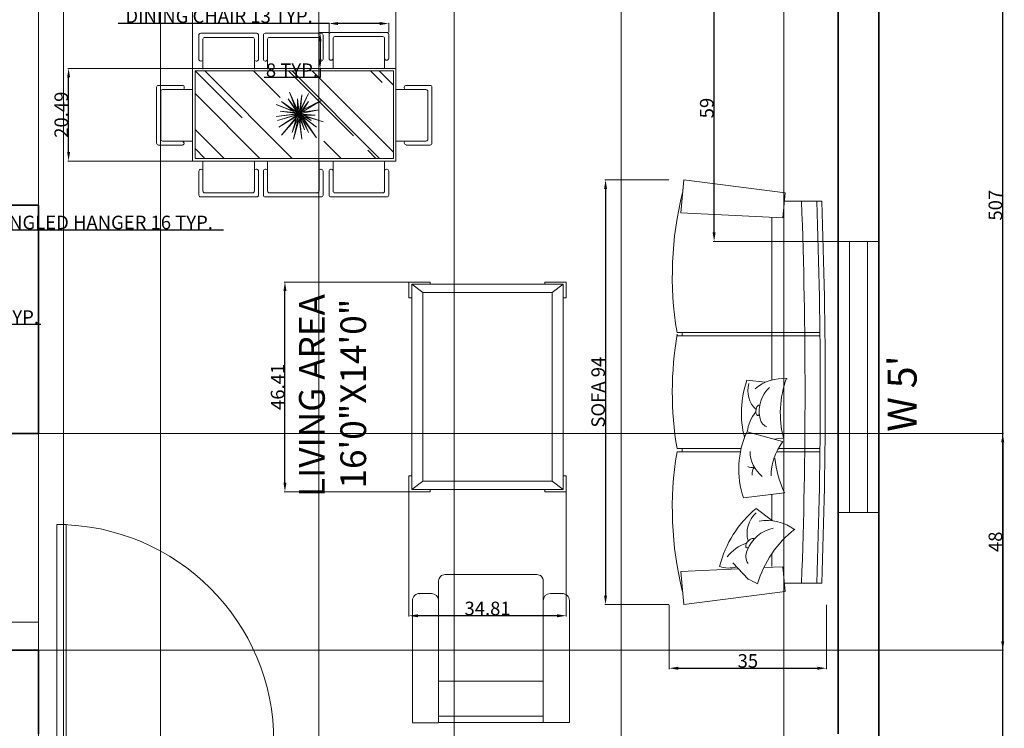
# Model space of a CAD drawing. Units: feet. Extents: x -297 to 770, y -228 to 625.
# Tile 5 of 14: x 552 to 770, y -62 to 95. Entities that reach past the tile are written whole.
import ezdxf

# ---------------------------------------------------------------- set-up
doc = ezdxf.new("R2010")
doc.units = ezdxf.units.FT
doc.header["$MEASUREMENT"] = 0
for name, color, linetype, lineweight in [('A-ANNO-DIMS', 2, 'Continuous', 18), ('A-ANNO-TEXT', 7, 'Continuous', 18), ('A-AREA-IDEN', 7, 'Continuous', 25), ('A-FURN', 8, 'Continuous', 18), ('A-WALL', 7, 'Continuous', 35), ('doors', 30, 'Continuous', 18), ('windows', 30, 'Continuous', 18)]:
    doc.layers.add(name, color=color, linetype=linetype, lineweight=lineweight)
doc.styles.add('Annotative', font='arial.ttf')
doc.styles.get("Standard").update_dxf_attribs({"font": 'arial.ttf'})
doc.dimstyles.get("Standard").update_dxf_attribs({"dimtxt": 3, "dimasz": 2, "dimexe": 0.18, "dimexo": 0.0625, "dimgap": 0.09, "dimtad": 1, "dimtoh": 1, "dimdec": 1, "dimzin": 0, "dimdsep": 46, "dimlunit": 3, "dimtxsty": 'Standard', "dimcen": 0, "dimclre": 256, "dimadec": 0, "dimazin": 0, "dimtfac": 1, "dimtdec": 1, "dimtofl": 0, "dimtmove": 0, "dimatfit": 3, "dimfxl": 1, "dimtolj": 1, "dimtzin": 0, "dimlwe": -1, "dimarcsym": 0})

# ---------------------------------------------------------------- blocks, each defined once
blk = doc.blocks.new('*U4')
for p, q in [((0, 0), (0, 6)), ((40, 0), (40, 6))]:
    blk.add_line(p, q)
blk.add_lwpolyline([(0, 0), (0, -40), (1.75, -40), (1.75, 0)], close=True)
blk.add_arc((0, 0), 40, 270, 0)
blk = doc.blocks.new('*U5')
for p, q in [((-40, 0), (-40, 6)), ((0, 0), (0, 6))]:
    blk.add_line(p, q)
blk.add_lwpolyline([(0, 0), (0, -40), (-1.75, -40), (-1.75, 0)], close=True)
blk.add_arc((0, 0), 40, 180, 270)
blk = doc.blocks.new('ММ404_2555х920')
for p, q in [((-1150, -20.9), (-1150, -245.9)), ((-360, -32.1), (-360, -892.6)), ((-340, -31.8), (-340, -892.6)), ((340, -31.8), (340, -283.8)), ((360, -32.1), (360, -293.8)), ((1150, -20.9), (1150, -245.9)), ((-1199.8, -241.6), (-1278.3, -852.1)), ((-1050.4, -254.7), (-1199.8, -241.6)), ((-1050.4, -254.7), (-1079.1, -869.5)), ((237.8, -471.1), (297.3, -256.4)), ((636.4, -491.8), (605.4, -246.1)), ((1050.4, -254.7), (1199.8, -241.6)), ((1050.4, -254.7), (1055.7, -369.5)), ((1199.8, -241.6), (1278.3, -852.1)), ((-1050, -320.9), (-73.8, -320.9)), ((614.8, -320.9), (774.2, -320.9)), ((699.6, -415.1), (774.5, -318.5)), ((971.6, -320.9), (1050, -320.9)), ((-72, -471.4), (-59.5, -361)), ((1026.9, -555.9), (1126.3, -464.2)), ((340, -506.7), (340, -892.6)), ((360, -511.1), (360, -892.6)), ((1062.9, -522.7), (1079.1, -869.5)), ((-1278.3, -852.1), (-1079.1, -869.5)), ((-360, -862.6), (-340, -862.6)), ((360, -862.6), (340, -862.6)), ((1278.3, -852.1), (1079.1, -869.5))]:
    blk.add_line(p, q)
for centre, radius, start, end in [((0, -31584.1), 31584.1, 87.91336, 92.08664), ((0, -31614.1), 31584.1, 87.91336, 92.08664), ((0, -31705.7), 31584.1, 87.91336, 92.08664), ((125.1, 326.1), 596.6, 249.48999, 284.83699), ((171.1, -255.4), 253.6, 174.21375, 221.17742), ((1051.5, -351.2), 279, 142.88134, 189.84501), ((1340.9, 221.6), 656.3, 218.15758, 253.50458), ((531.3, -258.2), 253.6, 178.2735, 191.49113), ((507.2, 23.9), 350.1, 233.17631, 269.54807), ((320.7, 386.4), 693.6, 276.31042, 294.23297), ((115.3, -200.3), 197.4, 223.39126, 280.29978), ((142.6, -321.2), 73.7, 276.25479, 334.78386), ((1030.6, -267.5), 217.1, 192.05885, 248.96737), ((85.8, -397.3), 8.22, 169.68836, 209.59655), ((85.8, -397.3), 8.22, 157.49693, 169.68836), ((98.3, -390.2), 22.6, 209.59655, 233.34145), ((108.2, -376.8), 39.2, 233.34145, 248.09558), ((117.3, -354.4), 63.4, 248.09558, 259.68836), ((122.4, -394.6), 22.6, 286.03528, 309.78017), ((119.1, -412.7), 22.6, 29.59655, 45.24399), ((131.6, -405.6), 8.22, 309.78017, 349.68836), ((131.6, -405.6), 8.22, 349.68836, 29.59655), ((353.1, -253.5), 199.6, 271.07138, 320.43697), ((1206.8, 1.3), 656.3, 219.38257, 256.10059), ((1388.4, -559.9), 279, 146.94109, 159.93675), ((125.1, 91.8), 596.6, 250.71498, 284.37724), ((-8.8, -312.1), 154, 253.94738, 317.31928), ((117.3, -354.4), 63.4, 259.68836, 271.28115), ((117.8, -378.6), 39.2, 271.28115, 286.03528), ((260.5, -254), 216.6, 229.12407, 264.09953), ((462.6, 9.9), 531, 244.94988, 289.10664), ((405.8, -444.2), 47.7, 332.00647, 20.30172), ((493.1, -362.9), 77.4, 236.70882, 274.52537), ((850, -301.6), 169.4, 222.61497, 285.98687), ((890.2, -435.7), 9.04, 138.35595, 178.26414), ((906, -436.2), 24.9, 178.26414, 202.00904), ((923, -429.3), 43.2, 202.00904, 216.76317), ((890.2, -435.7), 9.04, 126.16453, 138.35595), ((944.3, -413.4), 69.8, 216.76317, 228.35595), ((944.3, -413.4), 69.8, 228.35595, 239.94874), ((1136.3, -401), 238.2, 197.79166, 232.76712), ((931, -436.4), 43.2, 239.94874, 254.70287), ((928.5, -469.7), 9.04, 318.35595, 358.26414), ((912.6, -469.3), 24.9, 358.26414, 13.91158), ((987, -396.7), 81.1, 244.92238, 303.45145), ((926.1, -454.1), 24.9, 254.70287, 278.44776), ((928.5, -469.7), 9.04, 278.44776, 318.35595), ((896.2, -581.2), 162.4, 340.38592, 16.76075), ((-700, 1135.7), 2056.7, 255.87327, 279.51559), ((700, 1135.7), 2056.7, 260.48441, 284.12673), ((0, 1135.7), 2056.7, 260.20182, 279.51559)]:
    blk.add_arc(centre, radius, start, end)
blk = doc.blocks.new('WIN-5FT')
for p, q in [((60, 6.5), (0, 6.5)), ((60, 2.5), (0, 2.5))]:
    blk.add_line(p, q)
blk.add_lwpolyline([(60, 0), (60, 9), (0, 9), (0, 0)], close=True)
blk = doc.blocks.new('DINING-CHAIR')
for p, q in [((0.91, 1.32), (0.91, 7.97)), ((12.3, 7.97), (12.3, 1.32)), ((0, 0.41), (0, 5.72)), ((0.5, 6.13), (0.41, 6.13)), ((12.8, 6.13), (12.71, 6.13)), ((13.21, 5.72), (13.21, 0.41)), ((12.8, 0), (0.41, 0)), ((11.89, 0.91), (1.32, 0.91))]:
    blk.add_line(p, q)
for centre, start, end in [((0.41, 5.72), 90, 180), ((0.5, 5.72), 0, 90), ((12.71, 5.72), 90, 180), ((12.8, 5.72), 0, 90), ((0.41, 0.41), 180, 270), ((1.32, 1.32), 180, 270), ((11.89, 1.32), 270, 0), ((12.8, 0.41), 270, 0)]:
    blk.add_arc(centre, 0.41, start, end)
blk = doc.blocks.new('*D23')
at = {"layer": 'A-ANNO-DIMS', "transparency": 16777216}
for p, q in [((620.45, 91.75), (620.45, 93.85)), ((633.66, 91.75), (633.66, 93.85))]:
    blk.add_line(p, q, dxfattribs=at)
at = {"layer": 'A-ANNO-DIMS', "color": 0, "lineweight": -2, "transparency": 16777216}
for p, q in [((620.45, 93.67), (573.78, 93.67)), ((631.66, 93.67), (622.45, 93.67))]:
    blk.add_line(p, q, dxfattribs=at)
at = {"layer": 'A-ANNO-DIMS', "color": 0, "transparency": 16777216}
for points in [[(622.45, 94), (622.45, 93.33), (620.45, 93.67)], [(631.66, 94), (631.66, 93.33), (633.66, 93.67)]]:
    blk.add_solid(points, dxfattribs=at)
at = {"layer": 'Defpoints', "color": 0, "transparency": 16777216}
for p in [(620.45, 93.67), (620.45, 91.69), (633.66, 91.69)]:
    blk.add_point(p, dxfattribs=at)
at = {"layer": 'A-ANNO-DIMS', "color": 0, "transparency": 16777216, "insert": (596.11, 95.31), "char_height": 3, "attachment_point": 5}
blk.add_mtext('\\A1;DINING CHAIR 13 TYP.', dxfattribs=at)
blk = doc.blocks.new('*D24')
at = {"layer": 'A-ANNO-DIMS', "transparency": 16777216}
for p, q in [((620.39, 91.69), (618.29, 91.69)), ((620.39, 83.72), (618.29, 83.72))]:
    blk.add_line(p, q, dxfattribs=at)
at = {"layer": 'A-ANNO-DIMS', "color": 0, "lineweight": -2, "transparency": 16777216}
for p, q in [((618.47, 89.69), (618.47, 85.72)), ((618.47, 83.72), (618.47, 81.72)), ((618.47, 81.72), (606.1, 81.72))]:
    blk.add_line(p, q, dxfattribs=at)
at = {"layer": 'A-ANNO-DIMS', "color": 0, "transparency": 16777216}
for points in [[(618.14, 89.69), (618.8, 89.69), (618.47, 91.69)], [(618.14, 85.72), (618.8, 85.72), (618.47, 83.72)]]:
    blk.add_solid(points, dxfattribs=at)
at = {"layer": 'Defpoints', "color": 0, "transparency": 16777216}
for p in [(620.45, 91.69), (618.47, 83.72), (620.45, 83.72)]:
    blk.add_point(p, dxfattribs=at)
at = {"layer": 'A-ANNO-DIMS', "color": 0, "transparency": 16777216, "insert": (612.24, 83.34), "char_height": 3, "attachment_point": 5}
blk.add_mtext('\\A1;8 TYP.', dxfattribs=at)
blk = doc.blocks.new('*D33')
at = {"layer": 'A-ANNO-DIMS', "transparency": 16777216}
for p, q in [((695.7, 59.07), (681.49, 59.07)), ((695.7, -34.92), (681.49, -34.92))]:
    blk.add_line(p, q, dxfattribs=at)
at = {"layer": 'A-ANNO-DIMS', "color": 0, "lineweight": -2, "transparency": 16777216}
blk.add_line((681.67, 57.07), (681.67, -32.92), dxfattribs=at)
at = {"layer": 'A-ANNO-DIMS', "color": 0, "transparency": 16777216}
for points in [[(681.34, 57.07), (682, 57.07), (681.67, 59.07)], [(681.34, -32.92), (682, -32.92), (681.67, -34.92)]]:
    blk.add_solid(points, dxfattribs=at)
at = {"layer": 'Defpoints', "color": 0, "transparency": 16777216}
for p in [(695.77, 59.07), (681.67, -34.92), (695.77, -34.92)]:
    blk.add_point(p, dxfattribs=at)
at = {"layer": 'A-ANNO-DIMS', "color": 0, "transparency": 16777216, "insert": (680.03, 12.08), "char_height": 3, "attachment_point": 5, "rotation": 90}
blk.add_mtext('\\A1;SOFA 94', dxfattribs=at)
blk = doc.blocks.new('*D34')
at = {"layer": 'A-ANNO-DIMS', "transparency": 16777216}
for p, q in [((695.77, -34.98), (695.77, -49.19)), ((730.56, -34.98), (730.56, -49.19))]:
    blk.add_line(p, q, dxfattribs=at)
at = {"layer": 'A-ANNO-DIMS', "color": 0, "lineweight": -2, "transparency": 16777216}
blk.add_line((697.77, -49.01), (728.56, -49.01), dxfattribs=at)
at = {"layer": 'A-ANNO-DIMS', "color": 0, "transparency": 16777216}
for points in [[(697.77, -48.68), (697.77, -49.35), (695.77, -49.01)], [(728.56, -48.68), (728.56, -49.35), (730.56, -49.01)]]:
    blk.add_solid(points, dxfattribs=at)
at = {"layer": 'Defpoints', "color": 0, "transparency": 16777216}
for p in [(695.77, -34.92), (730.56, -34.92), (730.56, -49.01)]:
    blk.add_point(p, dxfattribs=at)
at = {"layer": 'A-ANNO-DIMS', "color": 0, "transparency": 16777216, "insert": (713.17, -47.39), "char_height": 3, "attachment_point": 5}
blk.add_mtext('\\A1;35', dxfattribs=at)
blk = doc.blocks.new('*D41')
at = {"layer": 'A-ANNO-DIMS', "color": 0, "lineweight": -2, "transparency": 16777216}
for p, q in [((544.72, 46), (544.72, 48)), ((544.72, 48), (597.08, 48)), ((544.72, 31.56), (544.72, 44))]:
    blk.add_line(p, q, dxfattribs=at)
at = {"layer": 'A-ANNO-DIMS', "transparency": 16777216}
for p, q in [((542.32, 46), (544.9, 46)), ((542.32, 29.56), (544.9, 29.56))]:
    blk.add_line(p, q, dxfattribs=at)
at = {"layer": 'A-ANNO-DIMS', "color": 0, "transparency": 16777216}
for points in [[(544.39, 44), (545.05, 44), (544.72, 46)], [(544.39, 31.56), (545.05, 31.56), (544.72, 29.56)]]:
    blk.add_solid(points, dxfattribs=at)
at = {"layer": 'Defpoints', "color": 0, "transparency": 16777216}
for p in [(542.25, 46), (544.72, 46), (542.25, 29.56)]:
    blk.add_point(p, dxfattribs=at)
at = {"layer": 'A-ANNO-DIMS', "color": 0, "transparency": 16777216, "insert": (570.94, 49.64), "char_height": 3, "attachment_point": 5}
blk.add_mtext('\\A1;ANGLED HANGER 16 TYP.', dxfattribs=at)
blk = doc.blocks.new('*D42')
at = {"layer": 'A-ANNO-DIMS', "transparency": 16777216}
for p, q in [((535.1, 29.5), (535.1, 26.92)), ((542.25, 29.5), (542.25, 26.92))]:
    blk.add_line(p, q, dxfattribs=at)
at = {"layer": 'A-ANNO-DIMS', "color": 0, "lineweight": -2, "transparency": 16777216}
for p, q in [((537.1, 27.1), (540.25, 27.1)), ((542.25, 27.1), (556.68, 27.1))]:
    blk.add_line(p, q, dxfattribs=at)
at = {"layer": 'A-ANNO-DIMS', "color": 0, "transparency": 16777216}
for points in [[(537.1, 27.43), (537.1, 26.76), (535.1, 27.1)], [(540.25, 27.43), (540.25, 26.76), (542.25, 27.1)]]:
    blk.add_solid(points, dxfattribs=at)
at = {"layer": 'Defpoints', "color": 0, "transparency": 16777216}
for p in [(535.1, 29.56), (542.25, 29.56), (542.25, 27.1)]:
    blk.add_point(p, dxfattribs=at)
at = {"layer": 'A-ANNO-DIMS', "color": 0, "transparency": 16777216, "insert": (550.47, 28.69), "char_height": 3, "attachment_point": 5}
blk.add_mtext('\\A1;7 TYP.', dxfattribs=at)
blk = doc.blocks.new('*D44')
at = {"layer": 'A-ANNO-DIMS', "transparency": 16777216}
for p, q in [((742.22, 306.96), (769.79, 306.96)), ((742.22, -200.04), (769.79, -200.04))]:
    blk.add_line(p, q, dxfattribs=at)
at = {"layer": 'A-ANNO-DIMS', "color": 0, "lineweight": -2, "transparency": 16777216}
blk.add_line((769.61, -198.04), (769.61, 304.96), dxfattribs=at)
at = {"layer": 'A-ANNO-DIMS', "color": 0, "transparency": 16777216}
for points in [[(769.27, 304.96), (769.94, 304.96), (769.61, 306.96)], [(769.27, -198.04), (769.94, -198.04), (769.61, -200.04)]]:
    blk.add_solid(points, dxfattribs=at)
at = {"layer": 'Defpoints', "color": 0, "transparency": 16777216}
for p in [(742.16, 306.96), (769.61, 306.96), (742.16, -200.04)]:
    blk.add_point(p, dxfattribs=at)
at = {"layer": 'A-ANNO-DIMS', "color": 0, "transparency": 16777216, "insert": (767.98, 53.46), "char_height": 3, "attachment_point": 5, "rotation": 90}
blk.add_mtext('\\A1;507', dxfattribs=at)
blk = doc.blocks.new('*D55')
at = {"layer": 'A-ANNO-DIMS', "transparency": 16777216}
for p, q in [((733.09, 104.46), (705.53, 104.46)), ((733.09, 45.46), (705.53, 45.46))]:
    blk.add_line(p, q, dxfattribs=at)
at = {"layer": 'A-ANNO-DIMS', "color": 0, "lineweight": -2, "transparency": 16777216}
blk.add_line((705.71, 47.46), (705.71, 102.46), dxfattribs=at)
at = {"layer": 'A-ANNO-DIMS', "color": 0, "transparency": 16777216}
for points in [[(705.37, 102.46), (706.04, 102.46), (705.71, 104.46)], [(705.37, 47.46), (706.04, 47.46), (705.71, 45.46)]]:
    blk.add_solid(points, dxfattribs=at)
at = {"layer": 'Defpoints', "color": 0, "transparency": 16777216}
for p in [(705.71, 104.46), (733.16, 104.46), (733.16, 45.46)]:
    blk.add_point(p, dxfattribs=at)
at = {"layer": 'A-ANNO-DIMS', "color": 0, "transparency": 16777216, "insert": (704.08, 74.96), "char_height": 3, "attachment_point": 5, "rotation": 90}
blk.add_mtext('\\A1;59', dxfattribs=at)
blk = doc.blocks.new('*D60')
at = {"layer": 'A-ANNO-DIMS', "transparency": 16777216}
for p, q in [((556.16, -144.47), (556.16, 367.22)), ((583.16, -144.47), (583.16, 367.22))]:
    blk.add_line(p, q, dxfattribs=at)
at = {"layer": 'A-ANNO-DIMS', "color": 0, "lineweight": -2, "transparency": 16777216}
blk.add_line((558.16, 367.04), (581.16, 367.04), dxfattribs=at)
at = {"layer": 'A-ANNO-DIMS', "color": 0, "transparency": 16777216}
for points in [[(558.16, 367.38), (558.16, 366.71), (556.16, 367.04)], [(581.16, 367.38), (581.16, 366.71), (583.16, 367.04)]]:
    blk.add_solid(points, dxfattribs=at)
at = {"layer": 'Defpoints', "color": 0, "transparency": 16777216}
for p in [(583.16, 367.04), (556.16, -144.54), (583.16, -144.54)]:
    blk.add_point(p, dxfattribs=at)
at = {"layer": 'A-ANNO-DIMS', "color": 0, "transparency": 16777216, "insert": (569.66, 368.64), "char_height": 3, "attachment_point": 5}
blk.add_mtext('\\A1;27', dxfattribs=at)
blk = doc.blocks.new('*D64')
at = {"layer": 'A-ANNO-DIMS', "transparency": 16777216}
for p, q in [((618.16, 233.4), (618.16, -227.67)), ((648.16, 233.4), (648.16, -227.67))]:
    blk.add_line(p, q, dxfattribs=at)
at = {"layer": 'A-ANNO-DIMS', "color": 0, "lineweight": -2, "transparency": 16777216}
blk.add_line((620.16, -227.49), (646.16, -227.49), dxfattribs=at)
at = {"layer": 'A-ANNO-DIMS', "color": 0, "transparency": 16777216}
for points in [[(620.16, -227.15), (620.16, -227.82), (618.16, -227.49)], [(646.16, -227.15), (646.16, -227.82), (648.16, -227.49)]]:
    blk.add_solid(points, dxfattribs=at)
at = {"layer": 'Defpoints', "color": 0, "transparency": 16777216}
for p in [(618.16, 233.46), (648.16, 233.46), (648.16, -227.49)]:
    blk.add_point(p, dxfattribs=at)
at = {"layer": 'A-ANNO-DIMS', "color": 0, "transparency": 16777216, "insert": (633.16, -225.86), "char_height": 3, "attachment_point": 5}
blk.add_mtext('\\A1;30', dxfattribs=at)
blk = doc.blocks.new('*D67')
at = {"layer": 'A-ANNO-DIMS', "transparency": 16777216}
for p, q in [((532.66, 197.4), (532.66, -227.67)), ((561.66, 197.4), (561.66, -227.67))]:
    blk.add_line(p, q, dxfattribs=at)
at = {"layer": 'A-ANNO-DIMS', "color": 0, "lineweight": -2, "transparency": 16777216}
blk.add_line((534.66, -227.49), (559.66, -227.49), dxfattribs=at)
at = {"layer": 'A-ANNO-DIMS', "color": 0, "transparency": 16777216}
for points in [[(534.66, -227.15), (534.66, -227.82), (532.66, -227.49)], [(559.66, -227.15), (559.66, -227.82), (561.66, -227.49)]]:
    blk.add_solid(points, dxfattribs=at)
at = {"layer": 'Defpoints', "color": 0, "transparency": 16777216}
for p in [(532.66, 197.46), (561.66, 197.46), (561.66, -227.49)]:
    blk.add_point(p, dxfattribs=at)
at = {"layer": 'A-ANNO-DIMS', "color": 0, "transparency": 16777216, "insert": (547.16, -225.87), "char_height": 3, "attachment_point": 5}
blk.add_mtext('\\A1;29', dxfattribs=at)
blk = doc.blocks.new('*D68')
at = {"layer": 'A-ANNO-DIMS', "transparency": 16777216}
for p, q in [((685.16, 306.9), (685.16, -227.67)), ((721.16, 306.9), (721.16, -227.67))]:
    blk.add_line(p, q, dxfattribs=at)
at = {"layer": 'A-ANNO-DIMS', "color": 0, "lineweight": -2, "transparency": 16777216}
blk.add_line((687.16, -227.49), (719.16, -227.49), dxfattribs=at)
at = {"layer": 'A-ANNO-DIMS', "color": 0, "transparency": 16777216}
for points in [[(687.16, -227.15), (687.16, -227.82), (685.16, -227.49)], [(719.16, -227.15), (719.16, -227.82), (721.16, -227.49)]]:
    blk.add_solid(points, dxfattribs=at)
at = {"layer": 'Defpoints', "color": 0, "transparency": 16777216}
for p in [(685.16, 306.96), (721.16, 306.96), (721.16, -227.49)]:
    blk.add_point(p, dxfattribs=at)
at = {"layer": 'A-ANNO-DIMS', "color": 0, "transparency": 16777216, "insert": (703.16, -225.86), "char_height": 3, "attachment_point": 5}
blk.add_mtext('\\A1;36', dxfattribs=at)
blk = doc.blocks.new('*D70')
at = {"layer": 'A-ANNO-DIMS', "transparency": 16777216}
for p, q in [((556.22, 2.96), (769.79, 2.96)), ((556.22, -45.04), (769.79, -45.04))]:
    blk.add_line(p, q, dxfattribs=at)
at = {"layer": 'A-ANNO-DIMS', "color": 0, "lineweight": -2, "transparency": 16777216}
blk.add_line((769.61, 0.96), (769.61, -43.04), dxfattribs=at)
at = {"layer": 'A-ANNO-DIMS', "color": 0, "transparency": 16777216}
for points in [[(769.27, 0.96), (769.94, 0.96), (769.61, 2.96)], [(769.27, -43.04), (769.94, -43.04), (769.61, -45.04)]]:
    blk.add_solid(points, dxfattribs=at)
at = {"layer": 'Defpoints', "color": 0, "transparency": 16777216}
for p in [(556.16, 2.96), (556.16, -45.04), (769.61, -45.04)]:
    blk.add_point(p, dxfattribs=at)
at = {"layer": 'A-ANNO-DIMS', "color": 0, "transparency": 16777216, "insert": (767.98, -21.04), "char_height": 3, "attachment_point": 5, "rotation": 90}
blk.add_mtext('\\A1;48', dxfattribs=at)
blk = doc.blocks.new('*D80')
at = {"layer": 'A-ANNO-DIMS', "transparency": 16777216}
for p, q in [((590.24, 83.79), (590.24, 111.36)), ((635.27, 83.79), (635.27, 111.36))]:
    blk.add_line(p, q, dxfattribs=at)
at = {"layer": 'A-ANNO-DIMS', "color": 0, "lineweight": -2, "transparency": 16777216}
blk.add_line((592.24, 111.18), (633.27, 111.18), dxfattribs=at)
at = {"layer": 'A-ANNO-DIMS', "color": 0, "transparency": 16777216}
for points in [[(592.24, 111.52), (592.24, 110.85), (590.24, 111.18)], [(633.27, 111.52), (633.27, 110.85), (635.27, 111.18)]]:
    blk.add_solid(points, dxfattribs=at)
at = {"layer": 'Defpoints', "color": 0, "transparency": 16777216}
for p in [(635.27, 111.18), (590.24, 83.73), (635.27, 83.73)]:
    blk.add_point(p, dxfattribs=at)
at = {"layer": 'A-ANNO-DIMS', "color": 0, "transparency": 16777216, "insert": (612.76, 112.81), "char_height": 3, "attachment_point": 5}
blk.add_mtext('\\A1;45.03', dxfattribs=at)
blk = doc.blocks.new('*D81')
at = {"layer": 'A-ANNO-DIMS', "transparency": 16777216}
for p, q in [((590.18, 83.73), (562.61, 83.73)), ((590.18, 63.24), (562.61, 63.24))]:
    blk.add_line(p, q, dxfattribs=at)
at = {"layer": 'A-ANNO-DIMS', "color": 0, "lineweight": -2, "transparency": 16777216}
blk.add_line((562.79, 65.24), (562.79, 81.73), dxfattribs=at)
at = {"layer": 'A-ANNO-DIMS', "color": 0, "transparency": 16777216}
for points in [[(562.46, 81.73), (563.12, 81.73), (562.79, 83.73)], [(562.46, 65.24), (563.12, 65.24), (562.79, 63.24)]]:
    blk.add_solid(points, dxfattribs=at)
at = {"layer": 'Defpoints', "color": 0, "transparency": 16777216}
for p in [(562.79, 83.73), (590.24, 83.73), (590.24, 63.24)]:
    blk.add_point(p, dxfattribs=at)
at = {"layer": 'A-ANNO-DIMS', "color": 0, "transparency": 16777216, "insert": (561.17, 73.49), "char_height": 3, "attachment_point": 5, "rotation": 90}
blk.add_mtext('\\A1;20.49', dxfattribs=at)
blk = doc.blocks.new('*D82')
at = {"layer": 'A-ANNO-DIMS', "transparency": 16777216}
for p, q in [((638.14, -10.01), (638.14, -37.58)), ((672.95, -10.01), (672.95, -37.58))]:
    blk.add_line(p, q, dxfattribs=at)
at = {"layer": 'A-ANNO-DIMS', "color": 0, "lineweight": -2, "transparency": 16777216}
blk.add_line((670.95, -37.4), (640.14, -37.4), dxfattribs=at)
at = {"layer": 'A-ANNO-DIMS', "color": 0, "transparency": 16777216}
for points in [[(640.14, -37.07), (640.14, -37.73), (638.14, -37.4)], [(670.95, -37.07), (670.95, -37.73), (672.95, -37.4)]]:
    blk.add_solid(points, dxfattribs=at)
at = {"layer": 'Defpoints', "color": 0, "transparency": 16777216}
for p in [(638.14, -9.95), (672.95, -9.95), (638.14, -37.4)]:
    blk.add_point(p, dxfattribs=at)
at = {"layer": 'A-ANNO-DIMS', "color": 0, "transparency": 16777216, "insert": (655.55, -35.78), "char_height": 3, "attachment_point": 5}
blk.add_mtext('\\A1;34.81', dxfattribs=at)
blk = doc.blocks.new('*D83')
at = {"layer": 'A-ANNO-DIMS', "transparency": 16777216}
for p, q in [((638.08, 36.46), (610.51, 36.46)), ((638.08, -9.95), (610.51, -9.95))]:
    blk.add_line(p, q, dxfattribs=at)
at = {"layer": 'A-ANNO-DIMS', "color": 0, "lineweight": -2, "transparency": 16777216}
blk.add_line((610.69, -7.95), (610.69, 34.46), dxfattribs=at)
at = {"layer": 'A-ANNO-DIMS', "color": 0, "transparency": 16777216}
for points in [[(610.36, 34.46), (611.02, 34.46), (610.69, 36.46)], [(610.36, -7.95), (611.02, -7.95), (610.69, -9.95)]]:
    blk.add_solid(points, dxfattribs=at)
at = {"layer": 'Defpoints', "color": 0, "transparency": 16777216}
for p in [(610.69, 36.46), (638.14, 36.46), (638.14, -9.95)]:
    blk.add_point(p, dxfattribs=at)
at = {"layer": 'A-ANNO-DIMS', "color": 0, "transparency": 16777216, "insert": (609.07, 13.26), "char_height": 3, "attachment_point": 5, "rotation": 90}
blk.add_mtext('\\A1;46.41', dxfattribs=at)

msp = doc.modelspace()

# ---------------------------------------------------------------- linework, layer by layer
at = {"layer": 'A-FURN'}
for p, q in [((590.239, 83.732), (590.239, 63.24)), ((635.271, 83.732), (590.239, 83.732)), ((590.809, 83.163), (590.809, 63.81)), ((634.702, 83.163), (590.809, 83.163)), ((601.211, 72.769), (590.817, 83.163)), ((612.296, 63.81), (592.943, 83.163)), ((609.615, 77.31), (603.762, 83.163)), ((625.844, 68.809), (611.49, 83.163)), ((631.616, 63.81), (612.263, 83.163)), ((634.702, 65.167), (616.706, 83.163)), ((632.22, 80.594), (629.651, 83.163)), ((634.702, 80.044), (631.583, 83.163)), ((634.702, 63.81), (634.702, 83.163)), ((635.271, 63.24), (635.271, 83.732)), ((582.273, 79.551), (582.273, 67.165)), ((587.988, 79.961), (582.682, 79.961)), ((583.183, 78.64), (583.183, 68.076)), ((590.239, 79.05), (583.593, 79.05)), ((588.398, 79.551), (588.398, 79.46)), ((635.271, 79.05), (641.917, 79.05)), ((637.113, 79.551), (637.113, 79.46)), ((637.523, 79.961), (642.828, 79.961)), ((642.327, 78.64), (642.327, 68.076)), ((643.238, 79.551), (643.238, 67.165)), ((605.148, 63.81), (590.809, 78.149)), ((613.805, 73.7), (609.938, 76.377)), ((612.615, 74.295), (609.938, 76.377)), ((613.805, 73.7), (611.425, 76.972)), ((611.425, 76.972), (613.21, 74.295)), ((613.805, 73.7), (611.722, 78.459)), ((611.722, 78.459), (613.21, 74.592)), ((613.805, 73.7), (613.507, 76.972)), ((613.507, 76.972), (613.507, 74.592)), ((613.805, 73.7), (615.887, 78.162)), ((613.805, 73.7), (614.4, 77.865)), ((613.805, 73.7), (618.862, 76.675)), ((613.805, 73.7), (615.887, 76.377)), ((614.102, 74.592), (615.887, 78.162)), ((614.4, 77.865), (614.102, 74.592)), ((615.887, 76.377), (614.452, 74.08)), ((618.862, 76.675), (614.805, 74.646)), ((615.887, 78.162), (615.887, 78.162)), ((613.805, 73.7), (608.748, 75.782)), ((608.748, 75.782), (612.615, 74.295)), ((609.64, 74.295), (612.912, 73.997)), ((613.805, 73.7), (609.64, 74.295)), ((613.805, 73.7), (618.267, 74.592)), ((618.267, 74.592), (614.452, 74.08)), ((608.748, 73.105), (613.21, 73.7)), ((613.805, 73.7), (608.748, 73.105)), ((613.805, 73.7), (609.045, 72.212)), ((609.045, 72.212), (613.21, 73.402)), ((613.805, 73.7), (609.343, 70.725)), ((609.343, 70.725), (613.21, 73.105)), ((613.805, 73.7), (609.938, 68.94)), ((609.938, 68.94), (613.147, 72.646)), ((613.805, 73.7), (612.317, 69.535)), ((612.317, 69.535), (613.147, 72.646)), ((613.805, 73.7), (612.615, 68.048)), ((613.805, 72.51), (612.615, 68.048)), ((613.805, 73.7), (614.4, 68.048)), ((613.805, 73.7), (617.375, 73.402)), ((613.805, 73.7), (615.887, 69.535)), ((613.805, 73.7), (614.995, 70.13)), ((613.805, 73.7), (617.672, 70.725)), ((613.805, 73.7), (616.482, 72.212)), ((613.805, 73.7), (617.672, 68.345)), ((613.805, 73.7), (619.16, 71.915)), ((614.4, 68.048), (613.805, 72.51)), ((614.995, 70.13), (613.89, 72.892)), ((617.672, 70.725), (614.102, 73.402)), ((617.375, 73.402), (614.697, 73.402)), ((617.672, 68.345), (614.697, 72.807)), ((615.887, 69.535), (614.738, 72.407)), ((616.482, 72.212), (615.292, 73.105)), ((619.16, 71.915), (615.292, 73.105)), ((597.226, 63.81), (590.809, 70.227)), ((583.593, 67.666), (590.239, 67.666)), ((623.115, 63.81), (619.275, 67.65)), ((641.917, 67.666), (635.271, 67.666)), ((582.682, 66.755), (587.988, 66.755)), ((588.398, 67.256), (588.398, 67.165)), ((592.976, 63.81), (590.809, 65.977)), ((630.843, 63.81), (629.032, 65.621)), ((637.113, 67.256), (637.113, 67.165)), ((642.828, 66.755), (637.523, 66.755)), ((590.239, 63.24), (635.271, 63.24)), ((590.809, 63.81), (634.702, 63.81)), ((638.141, 32.931), (638.141, 36.463)), ((638.141, 36.463), (642.827, 36.463)), ((638.811, 35.958), (641.252, 34.119)), ((638.811, 35.958), (672.281, 35.958)), ((638.811, -9.444), (638.811, 35.958)), ((642.827, 36.463), (642.827, 35.958)), ((668.264, 36.463), (672.95, 36.463)), ((668.264, 35.958), (668.264, 36.463)), ((669.839, 34.119), (672.281, 35.958)), ((672.281, 35.958), (672.281, -9.444)), ((672.95, 36.463), (672.95, 32.931)), ((638.811, 32.931), (638.141, 32.931)), ((641.252, 34.119), (641.252, -7.605)), ((669.839, 34.119), (641.252, 34.119)), ((669.839, -7.605), (669.839, 34.119)), ((672.95, 32.931), (672.281, 32.931)), ((638.141, -6.418), (638.811, -6.418)), ((638.141, -9.949), (638.141, -6.418)), ((672.281, -6.418), (672.95, -6.418)), ((672.95, -6.418), (672.95, -9.949)), ((641.252, -7.605), (638.811, -9.444)), ((641.252, -7.605), (669.839, -7.605)), ((672.281, -9.444), (669.839, -7.605)), ((642.827, -9.949), (638.141, -9.949)), ((672.281, -9.444), (638.811, -9.444)), ((642.827, -9.444), (642.827, -9.949)), ((668.264, -9.949), (668.264, -9.444)), ((672.95, -9.949), (668.264, -9.949)), ((666.459, -28.279), (646.125, -28.279)), ((644.716, -61.037), (644.716, -29.688)), ((667.867, -61.037), (667.867, -29.688)), ((643.118, -32.485), (640.526, -32.485)), ((669.465, -32.485), (672.057, -32.485)), ((638.928, -61.037), (638.928, -34.028)), ((673.655, -61.037), (673.655, -34.028)), ((667.867, -51.89), (644.716, -51.89)), ((667.867, -59.631), (644.716, -59.631)), ((638.929, -61.076), (644.716, -61.076)), ((673.655, -61.037), (644.716, -61.037))]:
    msp.add_line(p, q, dxfattribs=at)
for centre, radius, start, end in [((582.682, 79.551), 0.41, 90, 180), ((583.593, 78.64), 0.41, 90, 180), ((587.988, 79.551), 0.41, 0, 90), ((587.988, 79.46), 0.41, 270, 0), ((637.523, 79.551), 0.41, 90, 180), ((637.523, 79.46), 0.41, 180, 270), ((641.917, 78.64), 0.41, 0, 90), ((642.828, 79.551), 0.41, 0, 90), ((583.593, 68.076), 0.41, 180, 270), ((637.523, 67.256), 0.41, 90, 269.86312), ((641.917, 68.076), 0.41, 270, 0), ((582.682, 67.165), 0.41, 180, 270), ((587.988, 67.165), 0.41, 270, 90.05835), ((642.828, 67.165), 0.41, 270, 0), ((646.124, -29.688), 1.408, 89.99189, 180), ((666.459, -29.688), 1.408, 0, 90.00811), ((640.472, -34.028), 1.544, 88.00576, 180), ((643.118, -34.083), 1.598, 0, 90), ((669.465, -34.083), 1.598, 90, 180), ((672.111, -34.028), 1.544, 0, 91.99424)]:
    msp.add_arc(centre, radius, start, end, dxfattribs=at)
for p in [(640.526, -32.485), (672.057, -32.485)]:
    msp.add_point(p, dxfattribs=at)
at = {"layer": 'A-WALL'}
for p, q in [((742.155, -200.037), (742.155, 306.963)), ((391.155, 53.463), (556.155, 53.463)), ((556.155, 53.463), (556.155, 2.963)), ((547.155, 2.963), (556.155, 2.963)), ((547.155, -45.037), (556.155, -45.037)), ((556.155, -63.537), (556.155, -45.037))]:
    msp.add_line(p, q, dxfattribs=at)
msp.add_lwpolyline([(733.155, -63.537), (733.155, 104.463)], dxfattribs=at)

# ---------------------------------------------------------------- block references
at = {"layer": 'A-FURN', "rotation": 180}
for p in [(633.656, 91.685), (604.841, 91.5), (619.138, 91.5)]:
    msp.add_blockref('DINING-CHAIR', p, dxfattribs=at)
at = {"layer": 'A-FURN'}
for p in [(591.635, 55.287), (605.932, 55.287), (620.45, 55.287)]:
    msp.add_blockref('DINING-CHAIR', p, dxfattribs=at)
at = {"layer": 'A-FURN', "xscale": 0.0367624716155113, "yscale": 0.0367624716155113, "zscale": 0.0367624716155113, "rotation": 270}
msp.add_blockref('ММ404_2555х920', (730.308, 12.079), dxfattribs=at)
at = {"layer": 'doors'}
for name, p, xscale, yscale, zscale, rotation in [('*U4', (549.888, 2.963), 1.044609893629039, 1.044609893629039, 1.044609893629039, 270), ('*U5', (560.155, -65.322), 1.202549277038201, 1.202549277038201, 1.202549277038201, 180)]:
    msp.add_blockref(name, p, dxfattribs=dict(at, xscale=xscale, yscale=yscale, zscale=zscale, rotation=rotation))
at = {"layer": 'windows', "rotation": 90.00000000000003}
msp.add_blockref('WIN-5FT', (742.155, -14.537), dxfattribs=at)

# ---------------------------------------------------------------- texts
at = {"layer": 'A-ANNO-TEXT', "style": 'Annotative'}
msp.add_text("W 5'", height=6.4048, rotation=90, dxfattribs=at).set_placement((750.542, 3.316))
at = {"layer": 'A-AREA-IDEN', "style": 'Annotative'}
for s, p in [('LIVING AREA', (619.507, -11.126)), ('16\'0"X14\'0"', (628.657, -9.237))]:
    msp.add_text(s, height=5.69601, rotation=90, dxfattribs=at).set_placement(p)

# ---------------------------------------------------------------- dimensions: what is measured, and where the dimension line sits
at = {"layer": 'A-ANNO-DIMS'}
for base, p1, p2, override, picture, middle in [((583.155, 367.042), (556.155, -144.537), (583.155, -144.537), {"dimdec": 0, "dimlfac": 1, "dimrnd": 0, "dimzin": 0, "dimdsep": 46, "dimlunit": 2}, '*D60', (569.655, 368.638)), ((721.155, -227.487), (685.155, 306.963), (721.155, 306.963), {"dimdec": 0, "dimlfac": 1, "dimrnd": 0, "dimzin": 0, "dimdsep": 46, "dimlunit": 2}, '*D68', (703.155, -225.865)), ((648.155, -227.487), (618.155, 233.463), (648.155, 233.463), {"dimdec": 0, "dimlfac": 1, "dimrnd": 0, "dimzin": 0, "dimdsep": 46, "dimlunit": 2}, '*D64', (633.155, -225.865)), ((561.655, -227.487), (532.655, 197.463), (561.655, 197.463), {"dimdec": 0, "dimlfac": 1, "dimrnd": 0, "dimzin": 0, "dimdsep": 46, "dimlunit": 2}, '*D67', (547.155, -225.866)), ((635.271, 111.182), (590.239, 83.732), (635.271, 83.732), {"dimdec": 2, "dimlfac": 1, "dimrnd": 0, "dimzin": 0, "dimdsep": 46, "dimlunit": 2}, '*D80', (612.755, 112.805)), ((730.565, -49.014), (695.767, -34.916), (730.565, -34.916), {"dimdec": 0, "dimlfac": 1, "dimrnd": 0, "dimzin": 0, "dimdsep": 46, "dimlunit": 2}, '*D34', (713.166, -47.391))]:
    dim = msp.add_linear_dim(base=base, p1=p1, p2=p2, dimstyle='Standard', override=override, dxfattribs=at)
    dim.commit()
    dim.dimension.update_dxf_attribs({"geometry": picture, "text_midpoint": middle})
for base, p1, p2, angle, override, picture, middle in [((769.605, 306.963), (742.155, -200.037), (742.155, 306.963), 90, {"dimdec": 0, "dimlfac": 1, "dimrnd": 0, "dimzin": 0, "dimdsep": 46, "dimlunit": 2}, '*D44', (767.984, 53.463)), ((705.705, 104.463), (733.155, 45.463), (733.155, 104.463), 90, {"dimdec": 0, "dimlfac": 1, "dimrnd": 0, "dimzin": 0, "dimdsep": 46, "dimlunit": 2}, '*D55', (704.084, 74.963)), ((562.789, 83.732), (590.239, 63.24), (590.239, 83.732), 90, {"dimdec": 2, "dimlfac": 1, "dimrnd": 0, "dimzin": 0, "dimdsep": 46, "dimlunit": 2}, '*D81', (561.168, 73.486)), ((610.691, 36.463), (638.141, -9.949), (638.141, 36.463), 90, {"dimdec": 2, "dimlfac": 1, "dimrnd": 0, "dimzin": 0, "dimdsep": 46, "dimlunit": 2}, '*D83', (609.07, 13.257)), ((769.605, -45.037), (556.155, 2.963), (556.155, -45.037), 90, {"dimdec": 0, "dimlfac": 1, "dimrnd": 0, "dimzin": 0, "dimdsep": 46, "dimlunit": 2}, '*D70', (767.984, -21.037)), ((638.141, -37.399), (672.95, -9.949), (638.141, -9.949), 180, {"dimdec": 2, "dimlfac": 1, "dimrnd": 0, "dimzin": 0, "dimdsep": 46, "dimlunit": 2}, '*D82', (655.546, -35.776))]:
    dim = msp.add_linear_dim(base=base, p1=p1, p2=p2, angle=angle, dimstyle='Standard', override=override, dxfattribs=at)
    dim.commit()
    dim.dimension.update_dxf_attribs({"geometry": picture, "text_midpoint": middle})
for base, p1, p2, angle, text, picture, middle in [((620.45, 93.666), (633.656, 91.685), (620.45, 91.685), 180, 'DINING CHAIR <> TYP.', '*D23', (596.115, 95.309)), ((618.469, 83.719), (620.45, 91.685), (620.45, 83.719), 270, '<> TYP.', '*D24', (612.241, 83.341)), ((544.719, 46.003), (542.253, 29.562), (542.253, 46.003), 90, 'ANGLED HANGER <> TYP.', '*D41', (570.945, 49.644)), ((681.669, -34.916), (695.767, 59.073), (695.767, -34.916), 270, 'SOFA <>', '*D33', (680.027, 12.079))]:
    dim = msp.add_linear_dim(base=base, p1=p1, p2=p2, angle=angle, text=text, dimstyle='Standard', override={"dimdec": 0, "dimlfac": 1, "dimrnd": 0, "dimzin": 0, "dimdsep": 46, "dimlunit": 2}, dxfattribs=at)
    dim.commit()
    dim.dimension.update_dxf_attribs({"geometry": picture, "text_midpoint": middle})
dim = msp.add_linear_dim(base=(542.253, 27.096), p1=(535.099, 29.562), p2=(542.253, 29.562), text='<> TYP.', dimstyle='Standard', override={"dimdec": 0, "dimlfac": 1, "dimrnd": 0, "dimzin": 0, "dimdsep": 46, "dimlunit": 2}, dxfattribs=at)
dim.commit()
dim.dimension.update_dxf_attribs({"geometry": '*D42', "text_midpoint": (550.467, 28.687)})

doc.saveas('drawing.dxf')
